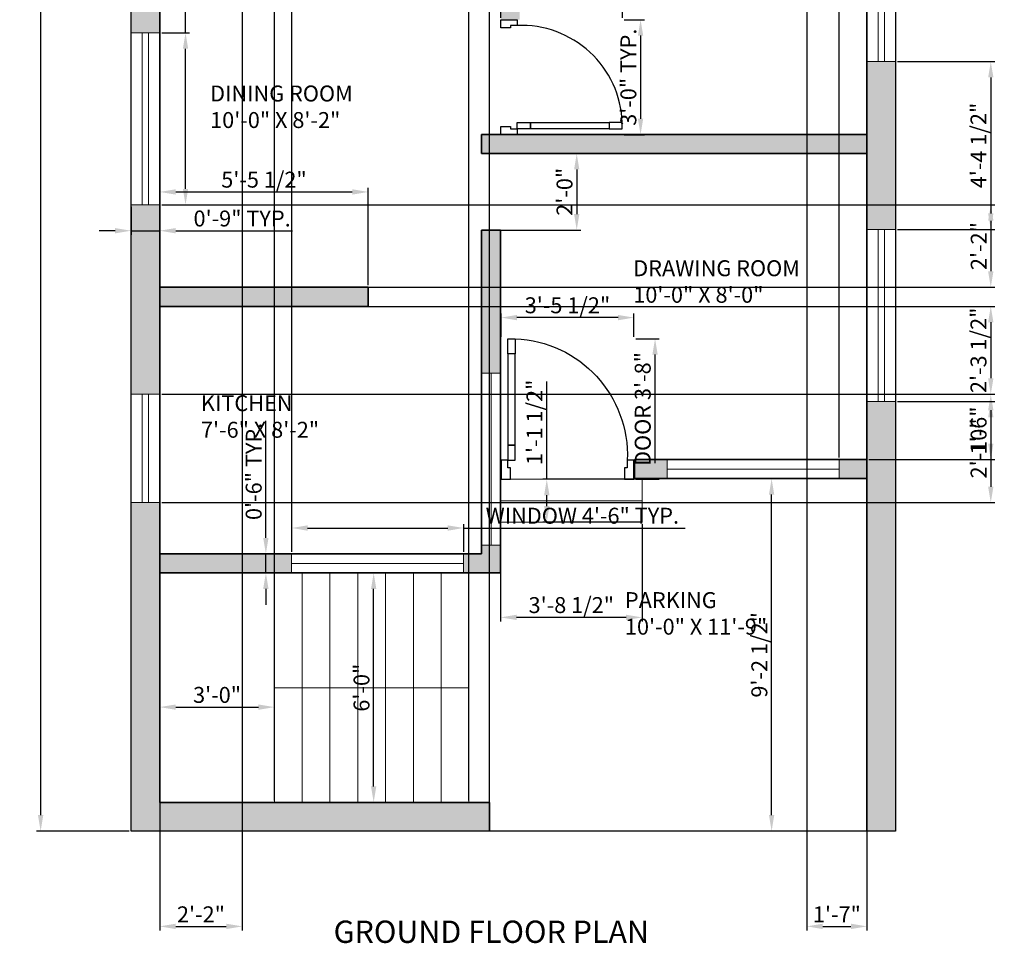
# Model space of a CAD drawing. Units: inches. Extents: x -32 to 277, y -560 to 55.
# Tile 1 of 2: x -32 to 277, y -560 to -271. Entities that reach past the tile are written whole.
import ezdxf

# ---------------------------------------------------------------- set-up
doc = ezdxf.new("R2010")
doc.units = ezdxf.units.IN
for name, color, linetype, lineweight in [('A-ANNO-DIMS', 2, 'Continuous', 18), ('A-ANNO-TEXT', 7, 'Continuous', 25), ('A-AREA-IDEN', 7, 'Continuous', 18), ('A-DOOR', 3, 'Continuous', 25), ('A-FLOR-STRS', 7, 'Continuous', 18), ('A-GLAZ', 4, 'Continuous', 18), ('A-WALL', 7, 'Continuous', 35), ('A-WALL-PATT', 252, 'Continuous', 13), ('C-PROP', 8, 'Continuous', 25)]:
    doc.layers.add(name, color=color, linetype=linetype, lineweight=lineweight)
doc.styles.get("Standard").update_dxf_attribs({"font": 'arial.ttf'})
doc.dimstyles.new('ISO-25', dxfattribs={"dimtxt": 5, "dimasz": 5, "dimexe": 1.25, "dimexo": 0.625, "dimtad": 1, "dimlunit": 3, "dimtxsty": 'Standard', "dimcen": 2.5, "dimadec": 0, "dimazin": 0, "dimtfac": 1, "dimtmove": 0, "dimatfit": 3, "dimfxl": 1, "dimarcsym": 0})

# ---------------------------------------------------------------- blocks, each defined once
blk = doc.blocks.new('A$C69F834CB')
for points in [[(625, 740), (625, 660), (665, 660), (665, 740)], [(625, 180), (625, 660), (665, 660), (665, 180)], [(625, 100), (625, 180), (665, 180), (665, 100)], [(35, 100), (35, 60), (50, 60), (50, 50), (50, 0), (0, 0), (0, 100)], [(665, 100), (700, 100), (700, 0), (650, 0), (650, 50), (650, 60), (665, 60)]]:
    blk.add_lwpolyline(points, close=True)
blk.add_arc((650, 125), 615.5, 92.3278, 182.3278)
blk = doc.blocks.new('*D3')
at = {"layer": 'A-ANNO-DIMS', "color": 0, "lineweight": -2, "transparency": 16777216}
for p, q in [((1.88, 14.77), (-27.13, 14.77)), ((-25.88, 9.77), (-25.88, -520.23)), ((1.88, -525.23), (-27.13, -525.23))]:
    blk.add_line(p, q, dxfattribs=at)
at = {"layer": 'A-ANNO-DIMS', "color": 0, "transparency": 16777216}
for points in [[(-26.72, 9.77), (-25.05, 9.77), (-25.88, 14.77)], [(-26.72, -520.23), (-25.05, -520.23), (-25.88, -525.23)]]:
    blk.add_solid(points, dxfattribs=at)
at = {"layer": 'Defpoints', "color": 0, "transparency": 16777216}
for p in [(2.51, 14.77), (-25.88, -525.23), (2.51, -525.23)]:
    blk.add_point(p, dxfattribs=at)
at = {"layer": 'A-ANNO-DIMS', "color": 0, "transparency": 16777216, "insert": (-29.05, -255.23), "char_height": 5, "attachment_point": 5, "rotation": 90}
blk.add_mtext("45'", dxfattribs=at)
blk = doc.blocks.new('WIN-54IN-9IN-WALL')
for p, q in [((3.5, 0), (3.5, 54)), ((5.5, 0), (5.5, 54))]:
    blk.add_line(p, q)
blk.add_lwpolyline([(9, 54), (9, 0), (0, 0), (0, 54)], close=True)
blk = doc.blocks.new('WIN-54IN-6IN-WALL')
blk.add_line((54, 3), (0, 3))
blk.add_lwpolyline([(0, 6), (54, 6), (54, 0), (0, 0)], close=True)
blk = doc.blocks.new('*D6')
at = {"layer": 'A-ANNO-DIMS', "color": 0, "lineweight": -2, "transparency": 16777216}
for p, q in [((19.61, -274.74), (19.61, -205.22)), ((12.13, -274.74), (20.86, -274.74)), ((19.61, -323.74), (19.61, -279.74)), ((12.13, -328.74), (20.86, -328.74))]:
    blk.add_line(p, q, dxfattribs=at)
at = {"layer": 'A-ANNO-DIMS', "color": 0, "transparency": 16777216}
for points in [[(18.78, -279.74), (20.44, -279.74), (19.61, -274.74)], [(18.78, -323.74), (20.44, -323.74), (19.61, -328.74)]]:
    blk.add_solid(points, dxfattribs=at)
at = {"layer": 'Defpoints', "color": 0, "transparency": 16777216}
for p in [(11.51, -274.74), (19.61, -274.74), (11.51, -328.74)]:
    blk.add_point(p, dxfattribs=at)
at = {"layer": 'A-ANNO-DIMS', "color": 0, "transparency": 16777216, "insert": (16.4, -237.48), "char_height": 5, "attachment_point": 5, "rotation": 90}
blk.add_mtext('WINDOW 4\'-6" TYP.', dxfattribs=at)
blk = doc.blocks.new('*D7')
at = {"layer": 'A-ANNO-DIMS', "color": 0, "lineweight": -2, "transparency": 16777216}
for p, q in [((2.51, -329.37), (2.51, -338.09)), ((11.51, -329.37), (11.51, -338.09)), ((-2.49, -336.84), (-7.49, -336.84)), ((2.51, -336.84), (11.51, -336.84)), ((16.51, -336.84), (53.24, -336.84))]:
    blk.add_line(p, q, dxfattribs=at)
at = {"layer": 'A-ANNO-DIMS', "color": 0, "transparency": 16777216}
for points in [[(-2.49, -336.01), (-2.49, -337.68), (2.51, -336.84)], [(16.51, -336.01), (16.51, -337.68), (11.51, -336.84)]]:
    blk.add_solid(points, dxfattribs=at)
at = {"layer": 'Defpoints', "color": 0, "transparency": 16777216}
for p in [(2.51, -328.74), (11.51, -328.74), (11.51, -336.84)]:
    blk.add_point(p, dxfattribs=at)
at = {"layer": 'A-ANNO-DIMS', "color": 0, "transparency": 16777216, "insert": (37.37, -333.66), "char_height": 5, "attachment_point": 5}
blk.add_mtext('0\'-9" TYP.', dxfattribs=at)
blk = doc.blocks.new('*D8')
at = {"layer": 'A-ANNO-DIMS', "color": 0, "lineweight": -2, "transparency": 16777216}
for p, q in [((52.93, -437.61), (52.93, -428.88)), ((106.93, -437.61), (106.93, -428.88)), ((57.93, -430.13), (101.93, -430.13)), ((106.93, -430.13), (176.45, -430.13))]:
    blk.add_line(p, q, dxfattribs=at)
at = {"layer": 'A-ANNO-DIMS', "color": 0, "transparency": 16777216}
for points in [[(57.93, -429.3), (57.93, -430.97), (52.93, -430.13)], [(101.93, -429.3), (101.93, -430.97), (106.93, -430.13)]]:
    blk.add_solid(points, dxfattribs=at)
at = {"layer": 'Defpoints', "color": 0, "transparency": 16777216}
for p in [(106.93, -430.13), (52.93, -438.23), (106.93, -438.23)]:
    blk.add_point(p, dxfattribs=at)
at = {"layer": 'A-ANNO-DIMS', "color": 0, "transparency": 16777216, "insert": (144.19, -426.92), "char_height": 5, "attachment_point": 5}
blk.add_mtext('WINDOW 4\'-6" TYP.', dxfattribs=at)
blk = doc.blocks.new('*D9')
at = {"layer": 'A-ANNO-DIMS', "color": 0, "lineweight": -2, "transparency": 16777216}
for p, q in [((44.83, -433.23), (44.83, -396.5)), ((52.3, -438.23), (43.58, -438.23)), ((44.83, -444.23), (44.83, -438.23)), ((52.3, -444.23), (43.58, -444.23)), ((44.83, -449.23), (44.83, -454.23))]:
    blk.add_line(p, q, dxfattribs=at)
at = {"layer": 'A-ANNO-DIMS', "color": 0, "transparency": 16777216}
for points in [[(43.99, -433.23), (45.66, -433.23), (44.83, -438.23)], [(43.99, -449.23), (45.66, -449.23), (44.83, -444.23)]]:
    blk.add_solid(points, dxfattribs=at)
at = {"layer": 'Defpoints', "color": 0, "transparency": 16777216}
for p in [(44.83, -438.23), (52.93, -438.23), (52.93, -444.23)]:
    blk.add_point(p, dxfattribs=at)
at = {"layer": 'A-ANNO-DIMS', "color": 0, "transparency": 16777216, "insert": (41.65, -412.37), "char_height": 5, "attachment_point": 5, "rotation": 90}
blk.add_mtext('0\'-6" TYP.', dxfattribs=at)
blk = doc.blocks.new('*D10')
at = {"layer": 'A-ANNO-DIMS', "color": 0, "lineweight": -2, "transparency": 16777216}
for p, q in [((118.58, -270.01), (118.58, -263.66)), ((123.58, -264.91), (151.74, -264.91)), ((156.74, -270.01), (156.74, -263.66)), ((156.74, -264.91), (216.11, -264.91))]:
    blk.add_line(p, q, dxfattribs=at)
at = {"layer": 'A-ANNO-DIMS', "color": 0, "transparency": 16777216}
for points in [[(123.58, -264.08), (123.58, -265.74), (118.58, -264.91)], [(151.74, -264.08), (151.74, -265.74), (156.74, -264.91)]]:
    blk.add_solid(points, dxfattribs=at)
at = {"layer": 'Defpoints', "color": 0, "transparency": 16777216}
for p in [(156.74, -264.91), (118.58, -270.63), (156.74, -270.63)]:
    blk.add_point(p, dxfattribs=at)
at = {"layer": 'A-ANNO-DIMS', "color": 0, "transparency": 16777216, "insert": (188.92, -261.7), "char_height": 5, "attachment_point": 5}
blk.add_mtext('DOOR 3\'-2" TYP.', dxfattribs=at)
blk = doc.blocks.new('*D11')
at = {"layer": 'A-ANNO-DIMS', "color": 0, "lineweight": -2, "transparency": 16777216}
for p, q in [((157.36, -270.63), (163.71, -270.63)), ((162.46, -275.63), (162.46, -301.72)), ((157.36, -306.72), (163.71, -306.72))]:
    blk.add_line(p, q, dxfattribs=at)
at = {"layer": 'A-ANNO-DIMS', "color": 0, "transparency": 16777216}
for points in [[(161.63, -275.63), (163.29, -275.63), (162.46, -270.63)], [(161.63, -301.72), (163.29, -301.72), (162.46, -306.72)]]:
    blk.add_solid(points, dxfattribs=at)
at = {"layer": 'Defpoints', "color": 0, "transparency": 16777216}
for p in [(156.74, -270.63), (156.74, -306.72), (162.46, -306.72)]:
    blk.add_point(p, dxfattribs=at)
at = {"layer": 'A-ANNO-DIMS', "color": 0, "transparency": 16777216, "insert": (159.28, -288.68), "char_height": 5, "attachment_point": 5, "rotation": 90}
blk.add_mtext('3\'-0" TYP.', dxfattribs=at)
blk = doc.blocks.new('*D16')
at = {"layer": 'A-ANNO-DIMS', "color": 0, "lineweight": -2, "transparency": 16777216}
for p, q in [((161.01, -370.72), (168.26, -370.72)), ((167.01, -409.83), (167.01, -375.72)), ((161.01, -414.83), (168.26, -414.83))]:
    blk.add_line(p, q, dxfattribs=at)
at = {"layer": 'A-ANNO-DIMS', "color": 0, "transparency": 16777216}
for points in [[(166.17, -375.72), (167.84, -375.72), (167.01, -370.72)], [(166.17, -409.83), (167.84, -409.83), (167.01, -414.83)]]:
    blk.add_solid(points, dxfattribs=at)
at = {"layer": 'Defpoints', "color": 0, "transparency": 16777216}
for p in [(160.39, -370.72), (167.01, -370.72), (160.39, -414.83)]:
    blk.add_point(p, dxfattribs=at)
at = {"layer": 'A-ANNO-DIMS', "color": 0, "transparency": 16777216, "insert": (163.79, -392.78), "char_height": 5, "attachment_point": 5, "rotation": 90}
blk.add_mtext('DOOR 3\'-8"', dxfattribs=at)
blk = doc.blocks.new('*D17')
at = {"layer": 'A-ANNO-DIMS', "color": 0, "lineweight": -2, "transparency": 16777216}
for p, q in [((118.66, -370.1), (118.66, -362.85)), ((155.39, -364.1), (123.66, -364.1)), ((160.39, -370.1), (160.39, -362.85))]:
    blk.add_line(p, q, dxfattribs=at)
at = {"layer": 'A-ANNO-DIMS', "color": 0, "transparency": 16777216}
for points in [[(123.66, -363.27), (123.66, -364.94), (118.66, -364.1)], [(155.39, -363.27), (155.39, -364.94), (160.39, -364.1)]]:
    blk.add_solid(points, dxfattribs=at)
at = {"layer": 'Defpoints', "color": 0, "transparency": 16777216}
for p in [(118.66, -364.1), (118.66, -370.72), (160.39, -370.72)]:
    blk.add_point(p, dxfattribs=at)
at = {"layer": 'A-ANNO-DIMS', "color": 0, "transparency": 16777216, "insert": (139.52, -360.89), "char_height": 5, "attachment_point": 5}
blk.add_mtext('3\'-5 1/2"', dxfattribs=at)
blk = doc.blocks.new('*D18')
at = {"layer": 'A-ANNO-DIMS', "color": 0, "lineweight": -2, "transparency": 16777216}
for p, q in [((11.51, 5.14), (11.51, -556.38)), ((37.4, 5.14), (37.4, -556.38)), ((16.51, -555.13), (32.4, -555.13))]:
    blk.add_line(p, q, dxfattribs=at)
at = {"layer": 'A-ANNO-DIMS', "color": 0, "transparency": 16777216}
for points in [[(16.51, -554.3), (16.51, -555.97), (11.51, -555.13)], [(32.4, -554.3), (32.4, -555.97), (37.4, -555.13)]]:
    blk.add_solid(points, dxfattribs=at)
at = {"layer": 'Defpoints', "color": 0, "transparency": 16777216}
for p in [(11.51, 5.77), (37.4, 5.77), (37.4, -555.13)]:
    blk.add_point(p, dxfattribs=at)
at = {"layer": 'A-ANNO-DIMS', "color": 0, "transparency": 16777216, "insert": (24.45, -552), "char_height": 5, "attachment_point": 5}
blk.add_mtext('2\'-2"', dxfattribs=at)
blk = doc.blocks.new('*D20')
at = {"layer": 'A-ANNO-DIMS', "color": 0, "lineweight": -2, "transparency": 16777216}
for p, q in [((214.66, 5.14), (214.66, -556.38)), ((233.51, 5.14), (233.51, -556.38)), ((219.66, -555.13), (228.51, -555.13))]:
    blk.add_line(p, q, dxfattribs=at)
at = {"layer": 'A-ANNO-DIMS', "color": 0, "transparency": 16777216}
for points in [[(219.66, -554.3), (219.66, -555.97), (214.66, -555.13)], [(228.51, -554.3), (228.51, -555.97), (233.51, -555.13)]]:
    blk.add_solid(points, dxfattribs=at)
at = {"layer": 'Defpoints', "color": 0, "transparency": 16777216}
for p in [(214.66, 5.77), (233.51, 5.77), (233.51, -555.13)]:
    blk.add_point(p, dxfattribs=at)
at = {"layer": 'A-ANNO-DIMS', "color": 0, "transparency": 16777216, "insert": (224.09, -552), "char_height": 5, "attachment_point": 5}
blk.add_mtext('1\'-7"', dxfattribs=at)
blk = doc.blocks.new('*D28')
at = {"layer": 'A-ANNO-DIMS', "color": 0, "lineweight": -2, "transparency": 16777216}
for p, q in [((243.13, -283.76), (273.66, -283.76)), ((272.41, -288.76), (272.41, -331.43)), ((243.13, -336.43), (273.66, -336.43))]:
    blk.add_line(p, q, dxfattribs=at)
at = {"layer": 'A-ANNO-DIMS', "color": 0, "transparency": 16777216}
for points in [[(271.58, -288.76), (273.25, -288.76), (272.41, -283.76)], [(271.58, -331.43), (273.25, -331.43), (272.41, -336.43)]]:
    blk.add_solid(points, dxfattribs=at)
at = {"layer": 'Defpoints', "color": 0, "transparency": 16777216}
for p in [(242.51, -283.76), (242.51, -336.43), (272.41, -336.43)]:
    blk.add_point(p, dxfattribs=at)
at = {"layer": 'A-ANNO-DIMS', "color": 0, "transparency": 16777216, "insert": (269.2, -310.1), "char_height": 5, "attachment_point": 5, "rotation": 90}
blk.add_mtext('4\'-4 1/2"', dxfattribs=at)
blk = doc.blocks.new('*D29')
at = {"layer": 'A-ANNO-DIMS', "color": 0, "lineweight": -2, "transparency": 16777216}
for p, q in [((243.13, -390.43), (273.66, -390.43)), ((272.41, -395.43), (272.41, -403.63)), ((234.13, -408.63), (273.66, -408.63))]:
    blk.add_line(p, q, dxfattribs=at)
at = {"layer": 'A-ANNO-DIMS', "color": 0, "transparency": 16777216}
for points in [[(271.58, -395.43), (273.25, -395.43), (272.41, -390.43)], [(271.58, -403.63), (273.25, -403.63), (272.41, -408.63)]]:
    blk.add_solid(points, dxfattribs=at)
at = {"layer": 'Defpoints', "color": 0, "transparency": 16777216}
for p in [(242.51, -390.43), (233.51, -408.63), (272.41, -408.63)]:
    blk.add_point(p, dxfattribs=at)
at = {"layer": 'A-ANNO-DIMS', "color": 0, "transparency": 16777216, "insert": (269.24, -399.53), "char_height": 5, "attachment_point": 5, "rotation": 90}
blk.add_mtext('1\'-6"', dxfattribs=at)
blk = doc.blocks.new('*D30')
at = {"layer": 'A-ANNO-DIMS', "color": 0, "lineweight": -2, "transparency": 16777216}
for p, q in [((232.88, -414.63), (202.36, -414.63)), ((203.61, -520.23), (203.61, -419.63)), ((232.88, -525.23), (202.36, -525.23))]:
    blk.add_line(p, q, dxfattribs=at)
at = {"layer": 'A-ANNO-DIMS', "color": 0, "transparency": 16777216}
for points in [[(202.78, -419.63), (204.44, -419.63), (203.61, -414.63)], [(202.78, -520.23), (204.44, -520.23), (203.61, -525.23)]]:
    blk.add_solid(points, dxfattribs=at)
at = {"layer": 'Defpoints', "color": 0, "transparency": 16777216}
for p in [(203.61, -414.63), (233.51, -414.63), (233.51, -525.23)]:
    blk.add_point(p, dxfattribs=at)
at = {"layer": 'A-ANNO-DIMS', "color": 0, "transparency": 16777216, "insert": (200.4, -469.93), "char_height": 5, "attachment_point": 5, "rotation": 90}
blk.add_mtext('9\'-2 1/2"', dxfattribs=at)
blk = doc.blocks.new('*D31')
at = {"layer": 'A-ANNO-DIMS', "color": 0, "lineweight": -2, "transparency": 16777216}
for p, q in [((12.13, -328.74), (273.66, -328.74)), ((272.41, -333.74), (272.41, -349.58)), ((12.13, -354.58), (273.66, -354.58))]:
    blk.add_line(p, q, dxfattribs=at)
at = {"layer": 'A-ANNO-DIMS', "color": 0, "transparency": 16777216}
for points in [[(271.58, -333.74), (273.25, -333.74), (272.41, -328.74)], [(271.58, -349.58), (273.25, -349.58), (272.41, -354.58)]]:
    blk.add_solid(points, dxfattribs=at)
at = {"layer": 'Defpoints', "color": 0, "transparency": 16777216}
for p in [(11.51, -328.74), (11.51, -354.58), (272.41, -354.58)]:
    blk.add_point(p, dxfattribs=at)
at = {"layer": 'A-ANNO-DIMS', "color": 0, "transparency": 16777216, "insert": (269.28, -341.66), "char_height": 5, "attachment_point": 5, "rotation": 90}
blk.add_mtext('2\'-2"', dxfattribs=at)
blk = doc.blocks.new('*D32')
at = {"layer": 'A-ANNO-DIMS', "color": 0, "lineweight": -2, "transparency": 16777216}
for p, q in [((11.51, -353.95), (11.51, -323.43)), ((76.97, -353.95), (76.97, -323.43)), ((16.51, -324.68), (71.97, -324.68))]:
    blk.add_line(p, q, dxfattribs=at)
at = {"layer": 'A-ANNO-DIMS', "color": 0, "transparency": 16777216}
for points in [[(16.51, -323.84), (16.51, -325.51), (11.51, -324.68)], [(71.97, -323.84), (71.97, -325.51), (76.97, -324.68)]]:
    blk.add_solid(points, dxfattribs=at)
at = {"layer": 'Defpoints', "color": 0, "transparency": 16777216}
for p in [(76.97, -324.68), (11.51, -354.58), (76.97, -354.58)]:
    blk.add_point(p, dxfattribs=at)
at = {"layer": 'A-ANNO-DIMS', "color": 0, "transparency": 16777216, "insert": (44.24, -321.47), "char_height": 5, "attachment_point": 5}
blk.add_mtext('5\'-5 1/2"', dxfattribs=at)
blk = doc.blocks.new('*D33')
at = {"layer": 'A-ANNO-DIMS', "color": 0, "lineweight": -2, "transparency": 16777216}
for p, q in [((113.15, -312.63), (143.67, -312.63)), ((142.42, -317.63), (142.42, -331.63)), ((113.15, -336.63), (143.67, -336.63))]:
    blk.add_line(p, q, dxfattribs=at)
at = {"layer": 'A-ANNO-DIMS', "color": 0, "transparency": 16777216}
for points in [[(141.59, -317.63), (143.25, -317.63), (142.42, -312.63)], [(141.59, -331.63), (143.25, -331.63), (142.42, -336.63)]]:
    blk.add_solid(points, dxfattribs=at)
at = {"layer": 'Defpoints', "color": 0, "transparency": 16777216}
for p in [(112.52, -312.63), (112.52, -336.63), (142.42, -336.63)]:
    blk.add_point(p, dxfattribs=at)
at = {"layer": 'A-ANNO-DIMS', "color": 0, "transparency": 16777216, "insert": (139.24, -324.63), "char_height": 5, "attachment_point": 5, "rotation": 90}
blk.add_mtext('2\'-0"', dxfattribs=at)
blk = doc.blocks.new('*D34')
at = {"layer": 'A-ANNO-DIMS', "color": 0, "lineweight": -2, "transparency": 16777216}
for p, q in [((12.13, -360.58), (273.66, -360.58)), ((272.41, -365.58), (272.41, -383.16)), ((12.13, -388.16), (273.66, -388.16))]:
    blk.add_line(p, q, dxfattribs=at)
at = {"layer": 'A-ANNO-DIMS', "color": 0, "transparency": 16777216}
for points in [[(271.58, -365.58), (273.25, -365.58), (272.41, -360.58)], [(271.58, -383.16), (273.25, -383.16), (272.41, -388.16)]]:
    blk.add_solid(points, dxfattribs=at)
at = {"layer": 'Defpoints', "color": 0, "transparency": 16777216}
for p in [(11.51, -360.58), (11.51, -388.16), (272.41, -388.16)]:
    blk.add_point(p, dxfattribs=at)
at = {"layer": 'A-ANNO-DIMS', "color": 0, "transparency": 16777216, "insert": (269.2, -374.37), "char_height": 5, "attachment_point": 5, "rotation": 90}
blk.add_mtext('2\'-3 1/2"', dxfattribs=at)
blk = doc.blocks.new('*D35')
at = {"layer": 'A-ANNO-DIMS', "color": 0, "lineweight": -2, "transparency": 16777216}
for p, q in [((12.13, -388.16), (273.66, -388.16)), ((272.41, -393.16), (272.41, -417.16)), ((12.13, -422.16), (273.66, -422.16))]:
    blk.add_line(p, q, dxfattribs=at)
at = {"layer": 'A-ANNO-DIMS', "color": 0, "transparency": 16777216}
for points in [[(271.58, -393.16), (273.25, -393.16), (272.41, -388.16)], [(271.58, -417.16), (273.25, -417.16), (272.41, -422.16)]]:
    blk.add_solid(points, dxfattribs=at)
at = {"layer": 'Defpoints', "color": 0, "transparency": 16777216}
for p in [(11.51, -388.16), (11.51, -422.16), (272.41, -422.16)]:
    blk.add_point(p, dxfattribs=at)
at = {"layer": 'A-ANNO-DIMS', "color": 0, "transparency": 16777216, "insert": (269.24, -405.16), "char_height": 5, "attachment_point": 5, "rotation": 90}
blk.add_mtext('2\'-10"', dxfattribs=at)
blk = doc.blocks.new('*D36')
at = {"layer": 'A-ANNO-DIMS', "color": 0, "lineweight": -2, "transparency": 16777216}
for p, q in [((107.95, -444.23), (77.42, -444.23)), ((78.67, -511.23), (78.67, -449.23)), ((107.95, -516.23), (77.42, -516.23))]:
    blk.add_line(p, q, dxfattribs=at)
at = {"layer": 'A-ANNO-DIMS', "color": 0, "transparency": 16777216}
for points in [[(77.84, -449.23), (79.51, -449.23), (78.67, -444.23)], [(77.84, -511.23), (79.51, -511.23), (78.67, -516.23)]]:
    blk.add_solid(points, dxfattribs=at)
at = {"layer": 'Defpoints', "color": 0, "transparency": 16777216}
for p in [(78.67, -444.23), (108.57, -444.23), (108.57, -516.23)]:
    blk.add_point(p, dxfattribs=at)
at = {"layer": 'A-ANNO-DIMS', "color": 0, "transparency": 16777216, "insert": (75.5, -480.23), "char_height": 5, "attachment_point": 5, "rotation": 90}
blk.add_mtext('6\'-0"', dxfattribs=at)
blk = doc.blocks.new('*D37')
at = {"layer": 'A-ANNO-DIMS', "color": 0, "lineweight": -2, "transparency": 16777216}
for p, q in [((11.51, -515.61), (11.51, -485.08)), ((47.51, -515.61), (47.51, -485.08)), ((16.51, -486.33), (42.51, -486.33))]:
    blk.add_line(p, q, dxfattribs=at)
at = {"layer": 'A-ANNO-DIMS', "color": 0, "transparency": 16777216}
for points in [[(16.51, -485.5), (16.51, -487.17), (11.51, -486.33)], [(42.51, -485.5), (42.51, -487.17), (47.51, -486.33)]]:
    blk.add_solid(points, dxfattribs=at)
at = {"layer": 'Defpoints', "color": 0, "transparency": 16777216}
for p in [(47.51, -486.33), (11.51, -516.23), (47.51, -516.23)]:
    blk.add_point(p, dxfattribs=at)
at = {"layer": 'A-ANNO-DIMS', "color": 0, "transparency": 16777216, "insert": (29.51, -483.15), "char_height": 5, "attachment_point": 5}
blk.add_mtext('3\'-0"', dxfattribs=at)
blk = doc.blocks.new('*D38')
at = {"layer": 'A-ANNO-DIMS', "color": 0, "lineweight": -2, "transparency": 16777216}
for p, q in [((47.51, -515.61), (47.51, 45.92)), ((52.51, 44.67), (103.57, 44.67)), ((108.57, -515.61), (108.57, 45.92))]:
    blk.add_line(p, q, dxfattribs=at)
at = {"layer": 'A-ANNO-DIMS', "color": 0, "transparency": 16777216}
for points in [[(52.51, 45.5), (52.51, 43.83), (47.51, 44.67)], [(103.57, 45.5), (103.57, 43.83), (108.57, 44.67)]]:
    blk.add_solid(points, dxfattribs=at)
at = {"layer": 'Defpoints', "color": 0, "transparency": 16777216}
for p in [(108.57, 44.67), (47.51, -516.23), (108.57, -516.23)]:
    blk.add_point(p, dxfattribs=at)
at = {"layer": 'A-ANNO-DIMS', "color": 0, "transparency": 16777216, "insert": (78.04, 47.85), "char_height": 5, "attachment_point": 5}
blk.add_mtext('5\'-1"', dxfattribs=at)
blk = doc.blocks.new('*D39')
at = {"layer": 'A-ANNO-DIMS', "color": 0, "lineweight": -2, "transparency": 16777216}
for p, q in [((114.99, -524.61), (114.99, 45.92)), ((119.99, 44.67), (228.51, 44.67)), ((233.51, -524.61), (233.51, 45.92))]:
    blk.add_line(p, q, dxfattribs=at)
at = {"layer": 'A-ANNO-DIMS', "color": 0, "transparency": 16777216}
for points in [[(119.99, 45.5), (119.99, 43.83), (114.99, 44.67)], [(228.51, 45.5), (228.51, 43.83), (233.51, 44.67)]]:
    blk.add_solid(points, dxfattribs=at)
at = {"layer": 'Defpoints', "color": 0, "transparency": 16777216}
for p in [(233.51, 44.67), (114.99, -525.23), (233.51, -525.23)]:
    blk.add_point(p, dxfattribs=at)
at = {"layer": 'A-ANNO-DIMS', "color": 0, "transparency": 16777216, "insert": (174.25, 47.88), "char_height": 5, "attachment_point": 5}
blk.add_mtext('9\'-10 1/2"', dxfattribs=at)
blk = doc.blocks.new('*D40')
at = {"layer": 'A-ANNO-DIMS', "color": 0, "lineweight": -2, "transparency": 16777216}
for p, q in [((11.51, -437.61), (11.51, 45.92)), ((16.51, 44.67), (47.93, 44.67)), ((52.93, -437.61), (52.93, 45.92))]:
    blk.add_line(p, q, dxfattribs=at)
at = {"layer": 'A-ANNO-DIMS', "color": 0, "transparency": 16777216}
for points in [[(16.51, 45.5), (16.51, 43.83), (11.51, 44.67)], [(47.93, 45.5), (47.93, 43.83), (52.93, 44.67)]]:
    blk.add_solid(points, dxfattribs=at)
at = {"layer": 'Defpoints', "color": 0, "transparency": 16777216}
for p in [(52.93, 44.67), (11.51, -438.23), (52.93, -438.23)]:
    blk.add_point(p, dxfattribs=at)
at = {"layer": 'A-ANNO-DIMS', "color": 0, "transparency": 16777216, "insert": (32.22, 47.88), "char_height": 5, "attachment_point": 5}
blk.add_mtext('3\'-5 1/2"', dxfattribs=at)
blk = doc.blocks.new('*D41')
at = {"layer": 'A-ANNO-DIMS', "color": 0, "lineweight": -2, "transparency": 16777216}
for p, q in [((219.85, 44.67), (214.85, 44.67)), ((224.85, -408), (224.85, 45.92)), ((224.85, 44.67), (233.51, 44.67)), ((233.51, -408), (233.51, 45.92)), ((238.51, 44.67), (269.7, 44.67))]:
    blk.add_line(p, q, dxfattribs=at)
at = {"layer": 'A-ANNO-DIMS', "color": 0, "transparency": 16777216}
for points in [[(219.85, 45.5), (219.85, 43.83), (224.85, 44.67)], [(238.51, 45.5), (238.51, 43.83), (233.51, 44.67)]]:
    blk.add_solid(points, dxfattribs=at)
at = {"layer": 'Defpoints', "color": 0, "transparency": 16777216}
for p in [(233.51, 44.67), (224.85, -408.63), (233.51, -408.63)]:
    blk.add_point(p, dxfattribs=at)
at = {"layer": 'A-ANNO-DIMS', "color": 0, "transparency": 16777216, "insert": (256.6, 47.88), "char_height": 5, "attachment_point": 5}
blk.add_mtext('0\'-8 1/2"', dxfattribs=at)
blk = doc.blocks.new('*D42')
at = {"layer": 'A-ANNO-DIMS', "color": 0, "lineweight": -2, "transparency": 16777216}
for p, q in [((118.52, -428.9), (118.52, -459.42)), ((162.92, -428.9), (162.92, -459.42)), ((157.92, -458.17), (123.52, -458.17))]:
    blk.add_line(p, q, dxfattribs=at)
at = {"layer": 'A-ANNO-DIMS', "color": 0, "transparency": 16777216}
for points in [[(123.52, -457.34), (123.52, -459), (118.52, -458.17)], [(157.92, -457.34), (157.92, -459), (162.92, -458.17)]]:
    blk.add_solid(points, dxfattribs=at)
at = {"layer": 'Defpoints', "color": 0, "transparency": 16777216}
for p in [(118.52, -428.27), (162.92, -428.27), (118.52, -458.17)]:
    blk.add_point(p, dxfattribs=at)
at = {"layer": 'A-ANNO-DIMS', "color": 0, "transparency": 16777216, "insert": (140.72, -454.96), "char_height": 5, "attachment_point": 5}
blk.add_mtext('3\'-8 1/2"', dxfattribs=at)
blk = doc.blocks.new('*D43')
at = {"layer": 'A-ANNO-DIMS', "color": 0, "lineweight": -2, "transparency": 16777216}
for p, q in [((133.02, -414.83), (133.02, -384.11)), ((162.3, -414.83), (131.77, -414.83)), ((133.02, -423.27), (133.02, -419.83)), ((162.3, -428.27), (131.77, -428.27))]:
    blk.add_line(p, q, dxfattribs=at)
at = {"layer": 'A-ANNO-DIMS', "color": 0, "transparency": 16777216}
for points in [[(132.19, -419.83), (133.86, -419.83), (133.02, -414.83)], [(132.19, -423.27), (133.86, -423.27), (133.02, -428.27)]]:
    blk.add_solid(points, dxfattribs=at)
at = {"layer": 'Defpoints', "color": 0, "transparency": 16777216}
for p in [(133.02, -414.83), (162.92, -414.83), (162.92, -428.27)]:
    blk.add_point(p, dxfattribs=at)
at = {"layer": 'A-ANNO-DIMS', "color": 0, "transparency": 16777216, "insert": (129.81, -396.97), "char_height": 5, "attachment_point": 5, "rotation": 90}
blk.add_mtext('1\'-1 1/2"', dxfattribs=at)

msp = doc.modelspace()

# ---------------------------------------------------------------- hatches: boundary and pattern name
at = {"layer": 'A-WALL-PATT'}
h = msp.add_hatch(color=256, dxfattribs=at)
h.dxf.hatch_style = 1
h.paths.add_polyline_path([(218.509, -120.232), (212.509, -120.232), (212.509, -180.252), (218.509, -180.252)])
h.paths.add_polyline_path([(164.509, -120.232), (158.509, -120.232), (158.509, -180.252), (164.509, -180.252)])
h.paths.add_polyline_path([(164.499, -114.232), (158.509, -114.232), (158.509, -120.232), (164.509, -120.232), (164.509, -118.512), (164.499, -118.512)])
h.paths.add_polyline_path([(65.509, -120.232), (59.509, -120.232), (59.509, -144.232), (11.509, -144.232), (11.509, -150.232), (59.509, -150.232), (65.509, -150.232)])
h.paths.add_polyline_path([(65.509, -180.281), (61.216, -180.281), (59.509, -180.232), (59.509, -228.232), (11.509, -228.232), (11.509, -234.232), (65.509, -234.232)])
h.paths.add_polyline_path([(11.509, -142.333), (2.509, -142.333), (2.509, -274.742), (11.509, -274.742)])
h = msp.add_hatch(color=256, dxfattribs=at)
h.dxf.hatch_style = 1
h.paths.add_polyline_path([(242.509, -180.232), (218.509, -180.252), (158.476, -180.252), (118.521, -180.696), (118.521, -186.63), (118.521, -270.63), (124.521, -270.63), (124.521, -186.63), (158.509, -186.252), (218.509, -186.252), (233.509, -186.24), (233.509, -229.761), (242.509, -229.761)])
h.paths.add_polyline_path([(242.509, -283.761), (233.509, -283.761), (233.509, -336.433), (242.509, -336.433)])
h.paths.add_polyline_path([(233.509, -306.63), (123.737, -306.63), (123.737, -306.725), (118.58, -306.725), (112.521, -306.63), (112.521, -312.63), (233.509, -312.63)])
h.paths.add_polyline_path([(11.509, -328.742), (2.509, -328.742), (2.509, -388.159), (11.509, -388.159)])
h.paths.add_polyline_path([(76.975, -354.577), (11.509, -354.577), (11.509, -360.577), (76.975, -360.577)])
h.paths.add_polyline_path([(118.521, -336.63), (112.521, -336.63), (112.521, -381.532), (118.521, -381.532)])
h.paths.add_polyline_path([(242.509, -390.433), (233.509, -390.433), (233.509, -516.232), (233.509, -525.232), (242.509, -525.232)])
h.paths.add_polyline_path([(233.509, -408.63), (224.849, -408.63), (224.849, -414.63), (233.509, -414.63)])
h.paths.add_polyline_path([(170.849, -408.63), (160.521, -408.63), (160.521, -414.63), (170.849, -414.63)])
h.paths.add_polyline_path([(118.521, -438.232), (118.521, -435.532), (112.521, -435.532), (112.521, -438.232), (106.925, -438.232), (106.925, -444.232), (113.551, -444.232), (118.521, -444.232)])
h.paths.add_polyline_path([(52.925, -438.232), (11.509, -438.232), (11.509, -444.232), (52.925, -444.232)], flags=17)
h.paths.add_polyline_path([(11.509, -444.232), (11.509, -422.159), (2.509, -422.159), (2.509, -525.232), (114.994, -525.232), (114.994, -516.232), (11.509, -516.232)])

# ---------------------------------------------------------------- linework, layer by layer
at = {"layer": 'A-FLOR-STRS'}
for p, q in [((162.923, -421.551), (118.521, -421.551)), ((47.509, -516.232), (47.509, -444.232)), ((56.232, -516.232), (56.232, -444.232)), ((64.956, -516.232), (64.956, -444.232)), ((73.679, -516.232), (73.679, -444.232)), ((82.403, -516.232), (82.403, -444.232)), ((91.126, -516.232), (91.126, -444.232)), ((99.85, -516.232), (99.85, -444.232)), ((108.573, -444.232), (108.573, -516.232)), ((108.573, -516.232), (108.573, -444.232)), ((47.509, -480.232), (108.573, -480.232))]:
    msp.add_line(p, q, dxfattribs=at)
msp.add_lwpolyline([(118.521, -414.832), (162.923, -414.832), (162.923, -428.271), (118.521, -428.271)], close=True, dxfattribs=at)
at = {"layer": 'A-GLAZ'}
for p, q in [((6.009, -388.159), (6.009, -422.159)), ((8.009, -388.159), (8.009, -422.159))]:
    msp.add_line(p, q, dxfattribs=at)
msp.add_lwpolyline([(2.509, -388.159), (11.509, -388.159), (11.509, -422.159), (2.509, -422.159)], close=True, dxfattribs=at)
at = {"layer": 'A-WALL'}
for p, q in [((11.509, -444.232), (11.509, 5.768)), ((233.509, -186.24), (233.509, -516.232)), ((112.521, -306.63), (233.509, -306.63)), ((112.521, -312.63), (112.521, -306.63)), ((124.521, -306.63), (118.521, -306.63)), ((112.521, -312.63), (233.509, -312.63)), ((112.521, -438.232), (112.521, -336.63)), ((112.521, -336.63), (118.521, -336.63)), ((118.521, -438.232), (118.521, -336.63)), ((76.975, -354.577), (11.509, -354.577)), ((76.975, -354.577), (76.975, -360.577)), ((76.975, -360.577), (11.509, -360.577)), ((118.521, -408.63), (118.521, -414.63)), ((160.521, -408.63), (233.509, -408.63)), ((160.521, -408.63), (160.521, -414.63)), ((160.521, -414.63), (233.509, -414.63)), ((11.509, -438.232), (112.521, -438.232)), ((118.521, -438.232), (118.521, -444.232)), ((11.509, -516.232), (11.509, -444.232)), ((11.509, -444.232), (113.551, -444.232)), ((113.551, -444.232), (118.521, -444.232)), ((114.994, -516.232), (11.509, -516.232)), ((114.994, -516.232), (114.994, -525.232)), ((233.509, -516.232), (233.509, -525.232))]:
    msp.add_line(p, q, dxfattribs=at)
at = {"layer": 'C-PROP'}
msp.add_lwpolyline([(2.509, 14.768), (242.509, 14.768), (242.509, -525.232), (2.509, -525.232)], close=True, dxfattribs=at)

# ---------------------------------------------------------------- block references
at = {"layer": 'A-DOOR', "xscale": 0.0515611792614383, "yscale": 0.0515611792614383, "zscale": 0.0515611792614383, "rotation": 270}
msp.add_blockref('A$C69F834CB', (118.58, -270.632), dxfattribs=at)
at = {"layer": 'A-DOOR', "xscale": -0.0596105960535776, "yscale": 0.0596105960535776, "zscale": 0.0596105960535776}
msp.add_blockref('A$C69F834CB', (160.388, -414.832), dxfattribs=at)
at = {"layer": 'A-GLAZ'}
for name, p in [('WIN-54IN-9IN-WALL', (233.509, -283.761)), ('WIN-54IN-9IN-WALL', (2.509, -328.742)), ('WIN-54IN-9IN-WALL', (233.509, -390.433)), ('WIN-54IN-6IN-WALL', (170.849, -414.63)), ('WIN-54IN-6IN-WALL', (52.926, -444.232))]:
    msp.add_blockref(name, p, dxfattribs=at)
at = {"layer": 'A-GLAZ', "rotation": 90.00000000000011}
msp.add_blockref('WIN-54IN-6IN-WALL', (118.521, -435.531), dxfattribs=at)

# ---------------------------------------------------------------- texts
at = {"layer": 'A-ANNO-TEXT', "insert": (66.089, -553.314), "char_height": 7, "attachment_point": 1}
msp.add_mtext_dynamic_manual_height_columns('GROUND FLOOR PLAN', width=255.40191, gutter_width=12.5, heights=[0], dxfattribs=at)
at = {"layer": 'A-AREA-IDEN', "char_height": 5, "attachment_point": 1}
for s, width, insert in [('DINING ROOM\\P10\'-0" X 8\'-2"', 64.54489, (27.324, -291.284)), ('DRAWING ROOM\\P10\'-0" X 8\'-0"', 65.22539, (160.169, -346.115)), ('KITCHEN\\P7\'-6" X 8\'-2"', 55.51621, (24.451, -388.463)), ('PARKING\\P10\'-0" X 11\'-9"', 55.8094, (157.548, -450.258))]:
    msp.add_mtext_dynamic_manual_height_columns(s, width=width, gutter_width=12.5, heights=[0], dxfattribs=dict(at, insert=insert))

# ---------------------------------------------------------------- dimensions: what is measured, and where the dimension line sits
at = {"layer": 'A-ANNO-DIMS'}
for base, p1, p2, picture, middle in [((52.925, 44.668), (11.509, -438.232), (52.925, -438.232), '*D40', (32.217, 47.88)), ((233.509, 44.668), (114.994, -525.232), (233.509, -525.232), '*D39', (174.252, 47.878)), ((233.509, 44.668), (224.849, -408.63), (233.509, -408.63), '*D41', (256.605, 47.878)), ((108.573, 44.668), (47.509, -516.232), (108.573, -516.232), '*D38', (78.041, 47.846)), ((37.398, -555.132), (11.509, 5.768), (37.398, 5.768), '*D18', (24.453, -551.997)), ((233.509, -555.132), (214.664, 5.768), (233.509, 5.768), '*D20', (224.087, -551.997)), ((76.975, -324.677), (11.509, -354.577), (76.975, -354.577), '*D32', (44.242, -321.467)), ((47.509, -486.332), (11.509, -516.232), (47.509, -516.232), '*D37', (29.509, -483.152))]:
    dim = msp.add_linear_dim(base=base, p1=p1, p2=p2, dimstyle='ISO-25', override={"dimdec": 1, "dimlfac": 1, "dimrnd": 0, "dimzin": 1, "dimdsep": 46, "dimlunit": 4, "dimfrac": 2}, dxfattribs=at)
    dim.commit()
    dim.dimension.update_dxf_attribs({"geometry": picture, "text_midpoint": middle})
for base, p1, p2, angle, override, picture, middle in [((-25.883, -525.232), (2.509, 14.768), (2.509, -525.232), 90, {"dimclrd": 0, "dimclre": 0, "dimclrt": 0}, '*D3', (-29.051, -255.232)), ((272.414, -336.433), (242.509, -283.761), (242.509, -336.433), 90, {"dimdec": 1, "dimlfac": 1, "dimrnd": 0, "dimzin": 1, "dimdsep": 46, "dimlunit": 4, "dimfrac": 2}, '*D28', (269.204, -310.097)), ((142.421, -336.63), (112.521, -312.63), (112.521, -336.63), 270, {"dimdec": 1, "dimlfac": 1, "dimrnd": 0, "dimzin": 1, "dimdsep": 46, "dimlunit": 4, "dimfrac": 2}, '*D33', (139.243, -324.63)), ((272.414, -354.577), (11.509, -328.742), (11.509, -354.577), 90, {"dimdec": 1, "dimlfac": 1, "dimrnd": 0, "dimzin": 1, "dimdsep": 46, "dimlunit": 4, "dimfrac": 2}, '*D31', (269.279, -341.66)), ((118.661, -364.103), (160.388, -370.72), (118.661, -370.72), 180, {"dimdec": 1, "dimlfac": 1, "dimrnd": 0, "dimzin": 1, "dimdsep": 46, "dimlunit": 4, "dimfrac": 2}, '*D17', (139.525, -360.891)), ((272.414, -388.159), (11.509, -360.577), (11.509, -388.159), 90, {"dimdec": 1, "dimlfac": 1, "dimrnd": 0, "dimzin": 1, "dimdsep": 46, "dimlunit": 4, "dimfrac": 2}, '*D34', (269.202, -374.368)), ((133.023, -414.832), (162.923, -428.271), (162.923, -414.832), 90, {"dimdec": 1, "dimlfac": 1, "dimrnd": 0, "dimzin": 1, "dimdsep": 46, "dimlunit": 4, "dimfrac": 2}, '*D43', (129.813, -396.971)), ((272.414, -422.159), (11.509, -388.159), (11.509, -422.159), 90, {"dimdec": 1, "dimlfac": 1, "dimrnd": 0, "dimzin": 1, "dimdsep": 46, "dimlunit": 4, "dimfrac": 2}, '*D35', (269.236, -405.159)), ((272.414, -408.63), (242.509, -390.433), (233.509, -408.63), 90, {"dimdec": 1, "dimlfac": 1, "dimrnd": 0, "dimzin": 1, "dimdsep": 46, "dimlunit": 4, "dimfrac": 2}, '*D29', (269.236, -399.532)), ((203.609, -414.63), (233.509, -525.232), (233.509, -414.63), 90, {"dimdec": 1, "dimlfac": 1, "dimrnd": 0, "dimzin": 1, "dimdsep": 46, "dimlunit": 4, "dimfrac": 2}, '*D30', (200.399, -469.931)), ((118.521, -458.171), (162.923, -428.271), (118.521, -428.271), 180, {"dimdec": 1, "dimlfac": 1, "dimrnd": 0, "dimzin": 1, "dimdsep": 46, "dimlunit": 4, "dimfrac": 2}, '*D42', (140.722, -454.959)), ((78.673, -444.232), (108.573, -516.232), (108.573, -444.232), 90, {"dimdec": 1, "dimlfac": 1, "dimrnd": 0, "dimzin": 1, "dimdsep": 46, "dimlunit": 4, "dimfrac": 2}, '*D36', (75.495, -480.232))]:
    dim = msp.add_linear_dim(base=base, p1=p1, p2=p2, angle=angle, dimstyle='ISO-25', override=override, dxfattribs=at)
    dim.commit()
    dim.dimension.update_dxf_attribs({"geometry": picture, "text_midpoint": middle})
for base, p1, p2, angle, text, picture, middle in [((19.609, -274.742), (11.509, -328.742), (11.509, -274.742), 90, 'WINDOW <> TYP.', '*D6', (16.397, -237.482)), ((162.459, -306.725), (156.736, -270.632), (156.736, -306.725), 270, '<> TYP.', '*D11', (159.279, -288.679)), ((167.005, -370.72), (160.388, -414.832), (160.388, -370.72), 90, 'DOOR <>', '*D16', (163.791, -392.776)), ((44.825, -438.232), (52.925, -444.232), (52.925, -438.232), 90, '<> TYP.', '*D9', (41.647, -412.368))]:
    dim = msp.add_linear_dim(base=base, p1=p1, p2=p2, angle=angle, text=text, dimstyle='ISO-25', override={"dimdec": 1, "dimlfac": 1, "dimrnd": 0, "dimzin": 1, "dimdsep": 46, "dimlunit": 4, "dimfrac": 2}, dxfattribs=at)
    dim.commit()
    dim.dimension.update_dxf_attribs({"geometry": picture, "text_midpoint": middle})
for base, p1, p2, text, picture, middle in [((156.736, -264.909), (118.58, -270.632), (156.736, -270.632), 'DOOR <> TYP.', '*D10', (188.923, -261.695)), ((11.509, -336.842), (2.509, -328.742), (11.509, -328.742), '<> TYP.', '*D7', (37.373, -333.664)), ((106.925, -430.132), (52.925, -438.232), (106.925, -438.232), 'WINDOW <> TYP.', '*D8', (144.186, -426.92))]:
    dim = msp.add_linear_dim(base=base, p1=p1, p2=p2, text=text, dimstyle='ISO-25', override={"dimdec": 1, "dimlfac": 1, "dimrnd": 0, "dimzin": 1, "dimdsep": 46, "dimlunit": 4, "dimfrac": 2}, dxfattribs=at)
    dim.commit()
    dim.dimension.update_dxf_attribs({"geometry": picture, "text_midpoint": middle})

doc.saveas('drawing.dxf')
